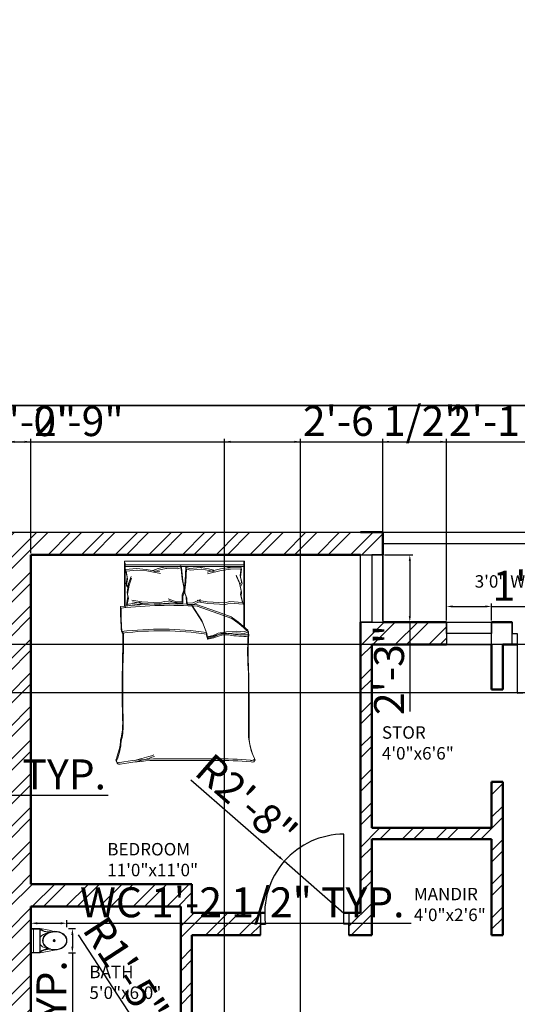
# Model space of a CAD drawing. Units: inches. Extents: x 1990 to 2869, y 1755 to 2533.
# Tile 5 of 6: x 2415 to 2615, y 2139 to 2533. Entities that reach past the tile are written whole.
import ezdxf

# ---------------------------------------------------------------- set-up
doc = ezdxf.new("R2010")
doc.units = ezdxf.units.IN
for name, color, linetype, lineweight in [('A-ANNO-DIMS', 171, 'Continuous', 18), ('A-ANNO-TTLB', 7, 'Continuous', 35), ('A-AREA-IDEN', 7, 'Continuous', 18), ('A-DOOR', 11, 'Continuous', 25), ('A-FLOR-FIXT', 9, 'Continuous', 20), ('A-FURN', 8, 'Continuous', 18), ('A-GLAZ', 121, 'Continuous', 25), ('A-WALL', 7, 'Continuous', 50), ('A-WALL-SITE', 7, 'Continuous', 30)]:
    doc.layers.add(name, color=color, linetype=linetype, lineweight=lineweight)
doc.layers.add('A-WALL-PATT', color=215, linetype='Continuous', lineweight=13, true_color=0xa953a0)
doc.styles.get("Standard").update_dxf_attribs({"font": 'arial.ttf'})
doc.dimstyles.new('ISO-25', dxfattribs={"dimtxt": 12, "dimasz": 2.5, "dimexe": 1.25, "dimexo": 0.625, "dimtad": 1, "dimdec": 0, "dimlunit": 3, "dimtxsty": 'Standard', "dimcen": 2.5, "dimadec": 0, "dimazin": 0, "dimtfac": 1, "dimtdec": 0, "dimtmove": 0, "dimatfit": 3, "dimfxl": 1, "dimarcsym": 0})

# ---------------------------------------------------------------- blocks, each defined once
blk = doc.blocks.new('A$C31115884')
for p, q in [((283, 498), (223, 498)), ((258, 466), (258, 523)), ((0, 200), (0, 0)), ((520, 200), (0, 200)), ((510, 54), (0, 54)), ((10, 190), (10, 10)), ((510, 190), (10, 190)), ((10, 10), (510, 10)), ((510, 10), (510, 190)), ((520, 0), (520, 200)), ((0, 0), (520, 0))]:
    blk.add_line(p, q)
blk.add_circle((256, 496), 23.6)
for centre, radius, start, end in [((2778, -205), 2807, 165.4549, 171.7133), ((-295, 403), 365, 324.2091, 9.3499), ((-295, 403), 375, 324.2091, 9.3499), ((806, 403), 365, 170.6501, 215.7909), ((3237, 905), 2807, 188.2867, 194.5451), ((384, 406), 293, 190.2774, 224.1564), ((139, 406), 293, 315.8436, 2.6563), ((806, 403), 375, 179.2036, 215.7909)]:
    blk.add_arc(centre, radius, start, end)
blk.add_ellipse((256, 510), major_axis=(0, -261), ratio=0.772727)
blk.add_open_spline([(256, 259), (263, 259), (270, 260), (288, 262), (299, 265), (320, 273), (330, 278), (350, 291), (360, 299), (378, 316), (386, 326), (402, 347), (409, 358), (421, 383), (427, 395), (436, 422), (440, 436), (445, 465), (447, 480), (448, 509), (448, 524), (445, 553), (443, 568), (436, 596), (432, 610), (422, 636), (416, 649), (402, 672), (395, 683), (379, 703), (370, 712), (351, 728), (341, 735), (321, 746), (310, 751), (289, 757), (278, 759), (256, 761), (245, 761), (223, 757), (212, 754), (191, 746), (181, 741), (161, 728), (151, 720), (133, 703), (125, 693), (110, 672), (103, 660), (90, 636), (85, 623), (76, 596), (72, 582), (67, 553), (66, 538), (64, 509), (65, 494), (68, 465), (70, 450), (77, 422), (81, 408), (91, 382), (97, 370), (111, 346), (118, 335), (135, 316), (144, 307), (162, 291), (172, 284), (193, 273), (203, 269), (225, 262), (236, 260), (250, 259), (253, 259), (256, 259)], degree=3, knots=[0, 0, 0, 0, 0.110105, 0.110105, 0.285049, 0.285049, 0.459994, 0.459994, 0.634938, 0.634938, 0.809882, 0.809882, 0.984827, 0.984827, 1.159771, 1.159771, 1.334715, 1.334715, 1.50966, 1.50966, 1.684604, 1.684604, 1.859549, 1.859549, 2.034493, 2.034493, 2.209437, 2.209437, 2.384382, 2.384382, 2.559326, 2.559326, 2.73427, 2.73427, 2.909215, 2.909215, 3.084159, 3.084159, 3.259103, 3.259103, 3.434048, 3.434048, 3.608992, 3.608992, 3.783936, 3.783936, 3.958881, 3.958881, 4.133825, 4.133825, 4.30877, 4.30877, 4.483714, 4.483714, 4.658658, 4.658658, 4.833603, 4.833603, 5.008547, 5.008547, 5.183491, 5.183491, 5.358436, 5.358436, 5.53338, 5.53338, 5.708324, 5.708324, 5.883269, 5.883269, 6.058213, 6.058213, 6.233158, 6.233158, 6.283185, 6.283185, 6.283185, 6.283185])
blk = doc.blocks.new('*D13')
at = {"layer": 'A-ANNO-DIMS', "color": 0, "lineweight": -2, "transparency": 16777216}
for p, q in [((2586.47, 2292.68), (2586.47, 2299.57)), ((2588.97, 2298.32), (2601.97, 2298.32)), ((2604.47, 2292.68), (2604.47, 2299.57)), ((2604.47, 2298.32), (2638.99, 2298.32))]:
    blk.add_line(p, q, dxfattribs=at)
at = {"layer": 'A-ANNO-DIMS', "color": 0, "transparency": 16777216}
for points in [[(2588.97, 2298.74), (2588.97, 2297.9), (2586.47, 2298.32)], [(2601.97, 2298.74), (2601.97, 2297.9), (2604.47, 2298.32)]]:
    blk.add_solid(points, dxfattribs=at)
at = {"layer": 'Defpoints', "color": 0, "transparency": 16777216}
for p in [(2604.47, 2298.32), (2586.47, 2292.05), (2604.47, 2292.05)]:
    blk.add_point(p, dxfattribs=at)
at = {"layer": 'A-ANNO-DIMS', "color": 0, "transparency": 16777216, "insert": (2622.98, 2305.07), "char_height": 12, "attachment_point": 5}
blk.add_mtext('1\'-6"', dxfattribs=at)
blk = doc.blocks.new('*D14')
at = {"layer": 'A-ANNO-DIMS', "color": 0, "lineweight": -2, "transparency": 16777216}
for p, q in [((2561.6, 2319.05), (2573, 2319.05)), ((2571.75, 2316.55), (2571.75, 2294.55)), ((2561.6, 2292.05), (2573, 2292.05)), ((2571.75, 2292.05), (2571.75, 2256.2))]:
    blk.add_line(p, q, dxfattribs=at)
at = {"layer": 'A-ANNO-DIMS', "color": 0, "transparency": 16777216}
for points in [[(2571.33, 2316.55), (2572.17, 2316.55), (2571.75, 2319.05)], [(2571.33, 2294.55), (2572.17, 2294.55), (2571.75, 2292.05)]]:
    blk.add_solid(points, dxfattribs=at)
at = {"layer": 'Defpoints', "color": 0, "transparency": 16777216}
for p in [(2560.97, 2319.05), (2560.97, 2292.05), (2571.75, 2292.05)]:
    blk.add_point(p, dxfattribs=at)
at = {"layer": 'A-ANNO-DIMS', "color": 0, "transparency": 16777216, "insert": (2564.99, 2272.87), "char_height": 12, "attachment_point": 5, "rotation": 90}
blk.add_mtext('2\'-3"', dxfattribs=at)
blk = doc.blocks.new('BED-DOUBLE')
for p, q in [((3.47, 63.33), (3.47, 81.44)), ((3.47, 81.44), (51.49, 81.44)), ((3.47, 79.91), (51.27, 79.91)), ((3.48, 63.33), (3.48, 81.44)), ((3.48, 79.91), (51.27, 79.91)), ((3.7, 62.69), (3.7, 80.8)), ((3.7, 62.69), (3.7, 80.8)), ((3.7, 79.27), (51.49, 79.27)), ((3.7, 79.27), (51.49, 79.27)), ((16.88, 78.42), (19.77, 79.14)), ((16.88, 78.42), (19.77, 79.14)), ((19.77, 79.14), (20.09, 79.14)), ((19.77, 79.14), (20.09, 79.14)), ((20.09, 79.14), (24.54, 78.99)), ((20.09, 79.14), (24.54, 78.99)), ((24.54, 78.99), (25.98, 79.57)), ((24.54, 78.99), (25.98, 79.57)), ((24.77, 78.36), (26.21, 78.93)), ((24.77, 78.36), (26.21, 78.93)), ((25.98, 79.57), (26.56, 74.22)), ((25.98, 79.57), (26.56, 74.22)), ((26.21, 78.93), (26.79, 73.58)), ((26.21, 78.93), (26.79, 73.58)), ((27.98, 78.95), (27.73, 73.58)), ((27.98, 78.95), (27.73, 73.58)), ((29.46, 78.46), (27.98, 78.95)), ((29.46, 78.46), (27.98, 78.95)), ((50.11, 78.89), (44.71, 78.98)), ((44.71, 78.98), (45.71, 78.9)), ((50.11, 78.89), (44.71, 78.98)), ((44.71, 78.98), (45.71, 78.9)), ((51.27, 81.44), (51.27, 54.83)), ((51.27, 81.44), (51.27, 54.83)), ((51.49, 81.44), (51.49, 80.8)), ((51.49, 80.8), (51.49, 54.19)), ((51.49, 80.8), (51.49, 54.19)), ((3.89, 78.13), (4.47, 74.95)), ((3.89, 78.13), (4.47, 74.95)), ((3.9, 78.11), (8.18, 78.43)), ((3.9, 78.11), (8.18, 78.43)), ((4.12, 77.49), (4.7, 74.31)), ((4.12, 77.49), (4.7, 74.31)), ((4.13, 77.47), (8.41, 77.8)), ((4.13, 77.47), (8.41, 77.8)), ((5.05, 72.49), (6.06, 75.24)), ((5.05, 72.49), (6.06, 75.24)), ((8.18, 78.43), (8.28, 78.42)), ((8.18, 78.43), (8.28, 78.42)), ((8.28, 78.42), (12.11, 78.13)), ((8.28, 78.42), (12.11, 78.13)), ((8.41, 77.8), (8.51, 77.78)), ((8.41, 77.8), (8.51, 77.78)), ((8.51, 77.78), (12.34, 77.49)), ((8.51, 77.78), (12.34, 77.49)), ((12.11, 78.13), (17.6, 77.11)), ((12.11, 78.13), (17.6, 77.11)), ((12.34, 77.49), (17.83, 76.48)), ((12.34, 77.49), (17.83, 76.48)), ((14.85, 77.69), (16.88, 78.42)), ((14.85, 77.69), (16.88, 78.42)), ((15.08, 77.05), (17.11, 77.78)), ((15.08, 77.05), (17.11, 77.78)), ((17.11, 77.78), (20, 78.5)), ((17.11, 77.78), (20, 78.5)), ((20, 78.5), (20.32, 78.5)), ((20, 78.5), (20.32, 78.5)), ((20.32, 78.5), (24.77, 78.36)), ((20.32, 78.5), (24.77, 78.36)), ((28.21, 78.31), (27.96, 72.94)), ((28.2, 78.31), (27.96, 72.94)), ((29.68, 77.82), (28.2, 78.31)), ((29.68, 77.82), (28.21, 78.31)), ((33.88, 78.89), (29.46, 78.46)), ((33.88, 78.89), (29.46, 78.46)), ((34.11, 78.25), (29.68, 77.82)), ((34.11, 78.25), (29.68, 77.82)), ((34.2, 78.91), (33.88, 78.89)), ((34.2, 78.91), (33.88, 78.89)), ((34.43, 78.27), (34.11, 78.25)), ((34.43, 78.27), (34.11, 78.25)), ((37.14, 78.36), (34.2, 78.91)), ((37.13, 78.36), (34.2, 78.91)), ((37.36, 77.73), (34.43, 78.27)), ((37.36, 77.73), (34.43, 78.27)), ((41.91, 78.37), (36.49, 77.02)), ((41.91, 78.37), (36.49, 77.02)), ((42.14, 77.73), (36.72, 76.38)), ((42.14, 77.73), (36.72, 76.38)), ((39.2, 77.77), (37.13, 78.36)), ((39.2, 77.77), (37.14, 78.36)), ((39.43, 77.13), (37.36, 77.73)), ((39.43, 77.13), (37.36, 77.73)), ((45.71, 78.9), (41.91, 78.37)), ((45.71, 78.9), (41.91, 78.37)), ((45.94, 78.26), (42.14, 77.73)), ((45.94, 78.26), (42.14, 77.73)), ((50.34, 78.25), (44.94, 78.34)), ((44.94, 78.34), (45.94, 78.26)), ((50.34, 78.25), (44.94, 78.34)), ((44.94, 78.34), (45.94, 78.26)), ((49.31, 73.19), (48.13, 75.86)), ((49.31, 73.19), (48.13, 75.86)), ((49.54, 72.55), (48.36, 75.23)), ((49.54, 72.55), (48.36, 75.23)), ((50.11, 78.89), (49.73, 75.68)), ((50.11, 78.89), (49.73, 75.68)), ((49.73, 75.68), (50.33, 73.1)), ((49.73, 75.68), (50.33, 73.1)), ((50.34, 78.25), (49.96, 75.04)), ((50.34, 78.25), (49.96, 75.04)), ((49.96, 75.04), (50.56, 72.47)), ((49.96, 75.04), (50.56, 72.47)), ((4.47, 74.95), (4.04, 72.34)), ((4.47, 74.95), (4.04, 72.34)), ((4.04, 72.34), (4.62, 71.33)), ((4.04, 72.34), (4.62, 71.33)), ((4.7, 74.31), (4.27, 71.7)), ((4.7, 74.31), (4.27, 71.7)), ((4.27, 71.7), (4.85, 70.69)), ((4.27, 71.7), (4.85, 70.69)), ((4.47, 68.87), (5.05, 72.49)), ((4.47, 68.87), (5.05, 72.49)), ((4.7, 68.23), (5.28, 71.85)), ((4.7, 68.23), (5.28, 71.85)), ((5.28, 71.85), (6.29, 74.6)), ((5.28, 71.85), (6.29, 74.6)), ((26.56, 74.22), (27.14, 71.04)), ((26.56, 74.22), (27.14, 71.04)), ((26.79, 73.58), (27.37, 70.4)), ((26.79, 73.58), (27.37, 70.4)), ((27.14, 71.04), (27.14, 69.74)), ((27.14, 71.04), (27.14, 69.74)), ((27.73, 73.58), (27.35, 70.37)), ((27.73, 73.58), (27.35, 70.37)), ((27.96, 72.94), (27.58, 69.73)), ((27.96, 72.94), (27.58, 69.73)), ((50.11, 69.61), (49.31, 73.19)), ((50.11, 69.61), (49.31, 73.19)), ((50.34, 68.98), (49.54, 72.55)), ((50.34, 68.98), (49.54, 72.55)), ((50.33, 73.1), (49.81, 72.06)), ((50.33, 73.1), (49.81, 72.06)), ((50.56, 72.47), (50.04, 71.42)), ((50.56, 72.47), (50.04, 71.42)), ((4.18, 64.1), (4.76, 67.28)), ((4.18, 64.1), (4.76, 67.28)), ((4.76, 67.28), (4.47, 68.87)), ((4.76, 67.28), (4.47, 68.87)), ((4.99, 66.64), (4.7, 68.23)), ((4.99, 66.64), (4.7, 68.23)), ((27.14, 69.74), (26.56, 67.86)), ((27.14, 69.74), (26.56, 67.86)), ((26.56, 67.86), (26.56, 65.18)), ((26.56, 67.86), (26.56, 65.18)), ((27.37, 69.1), (26.79, 67.22)), ((27.37, 69.1), (26.79, 67.22)), ((26.79, 67.22), (26.79, 64.54)), ((26.79, 67.22), (26.79, 64.54)), ((27.35, 70.37), (27.44, 69.07)), ((27.35, 70.37), (27.44, 69.07)), ((27.37, 70.4), (27.37, 69.1)), ((27.37, 70.4), (27.37, 69.1)), ((27.44, 69.07), (28.13, 67.23)), ((27.44, 69.07), (28.13, 67.23)), ((27.58, 69.73), (27.66, 68.43)), ((27.58, 69.73), (27.66, 68.43)), ((27.66, 68.43), (28.36, 66.59)), ((27.66, 68.43), (28.36, 66.59)), ((28.13, 67.23), (28.3, 64.55)), ((28.13, 67.23), (28.3, 64.55)), ((49.92, 68.01), (50.11, 69.61)), ((49.92, 68.01), (50.11, 69.61)), ((50.7, 64.87), (49.92, 68.01)), ((50.7, 64.87), (49.92, 68.01)), ((50.15, 67.37), (50.34, 68.98)), ((50.15, 67.37), (50.34, 68.98)), ((50.93, 64.23), (50.15, 67.37)), ((50.93, 64.23), (50.15, 67.37)), ((9.28, 64.82), (4.18, 64.1)), ((9.28, 64.82), (4.18, 64.1)), ((4.41, 63.46), (4.99, 66.64)), ((4.41, 63.46), (4.99, 66.64)), ((9.51, 64.19), (4.41, 63.46)), ((9.51, 64.19), (4.41, 63.46)), ((6.38, 65.81), (10.41, 65.15)), ((6.38, 65.81), (10.41, 65.15)), ((6.61, 65.18), (10.64, 64.51)), ((6.61, 65.18), (10.64, 64.51)), ((10.41, 65.15), (9.28, 64.82)), ((10.41, 65.15), (9.28, 64.82)), ((10.64, 64.51), (9.51, 64.19)), ((10.64, 64.51), (9.51, 64.19)), ((10.41, 65.15), (17.42, 64.72)), ((10.41, 65.15), (17.42, 64.72)), ((10.64, 64.51), (17.65, 64.08)), ((10.64, 64.51), (17.65, 64.08)), ((17.42, 64.72), (19.38, 65.27)), ((17.42, 64.72), (19.38, 65.27)), ((17.65, 64.08), (19.61, 64.63)), ((17.65, 64.08), (19.61, 64.63)), ((19.38, 65.27), (24.52, 64.87)), ((19.38, 65.27), (24.52, 64.87)), ((19.61, 64.63), (24.74, 64.23)), ((19.61, 64.63), (24.74, 64.23)), ((24.1, 65.18), (20.96, 66.27)), ((24.1, 65.18), (20.96, 66.27)), ((24.33, 64.54), (21.19, 65.63)), ((24.33, 64.54), (21.19, 65.63)), ((26.56, 65.18), (24.1, 65.18)), ((26.56, 65.18), (24.1, 65.18)), ((26.79, 64.54), (24.33, 64.54)), ((26.79, 64.54), (24.33, 64.54)), ((28.3, 64.55), (30.75, 64.7)), ((28.3, 64.55), (30.75, 64.7)), ((28.36, 66.59), (28.53, 63.91)), ((28.36, 66.59), (28.53, 63.91)), ((28.53, 63.91), (30.98, 64.06)), ((28.53, 63.91), (30.98, 64.06)), ((30.26, 64.06), (34.45, 57.57)), ((30.26, 64.06), (34.45, 57.57)), ((30.49, 63.42), (34.68, 56.93)), ((30.49, 63.42), (34.68, 56.93)), ((30.75, 64.7), (33.82, 65.99)), ((30.75, 64.7), (33.82, 65.99)), ((30.98, 64.06), (34.05, 65.35)), ((30.98, 64.06), (34.05, 65.35)), ((40.64, 61.13), (32.31, 64.06)), ((40.64, 61.13), (32.31, 64.06)), ((40.87, 60.49), (32.53, 63.42)), ((40.87, 60.49), (32.53, 63.42)), ((32.56, 65.81), (36.6, 65.15)), ((32.56, 65.81), (36.6, 65.15)), ((32.79, 65.18), (36.82, 64.51)), ((32.79, 65.18), (36.82, 64.51)), ((36.6, 65.15), (43.61, 64.72)), ((36.6, 65.15), (43.61, 64.72)), ((36.82, 64.51), (43.83, 64.08)), ((36.82, 64.51), (43.83, 64.08)), ((43.61, 64.72), (45.57, 65.27)), ((43.61, 64.72), (45.57, 65.27)), ((43.83, 64.08), (45.79, 64.63)), ((43.83, 64.08), (45.79, 64.63)), ((45.57, 65.27), (50.7, 64.87)), ((45.57, 65.27), (50.7, 64.87)), ((45.79, 64.63), (50.93, 64.23)), ((45.79, 64.63), (50.93, 64.23)), ((46.22, 59.11), (40.64, 61.13)), ((46.22, 59.11), (40.64, 61.13)), ((46.45, 58.48), (40.87, 60.49)), ((46.45, 58.48), (40.87, 60.49)), ((34.45, 57.57), (36.15, 53.08)), ((34.45, 57.57), (36.15, 53.08)), ((34.68, 56.93), (36.38, 52.44)), ((34.68, 56.93), (36.38, 52.44)), ((49.16, 56.95), (46.22, 59.11)), ((49.16, 56.95), (46.22, 59.11)), ((49.39, 56.31), (46.45, 58.48)), ((49.39, 56.31), (46.45, 58.48)), ((52.87, 53.7), (49.16, 56.95)), ((52.87, 53.7), (49.16, 56.95)), ((53.1, 53.06), (49.39, 56.31)), ((53.1, 53.06), (49.39, 56.31)), ((36.15, 53.08), (36.46, 51.07)), ((36.15, 53.08), (36.46, 51.07)), ((36.38, 52.44), (36.69, 50.43)), ((36.38, 52.44), (36.69, 50.43)), ((36.46, 51.07), (38.94, 51.69)), ((36.46, 51.07), (38.94, 51.69)), ((38.94, 51.69), (40.95, 52.61)), ((38.94, 51.69), (40.95, 52.61)), ((39.17, 51.05), (41.18, 51.97)), ((39.17, 51.05), (41.18, 51.97)), ((40.95, 52.61), (44.36, 53.08)), ((40.95, 52.61), (44.36, 53.08)), ((41.18, 51.97), (44.59, 52.44)), ((41.18, 51.97), (44.59, 52.44)), ((44.36, 53.08), (48.23, 53.39)), ((44.36, 53.08), (48.23, 53.39)), ((44.59, 52.44), (48.46, 52.75)), ((44.59, 52.44), (48.46, 52.75)), ((48.23, 53.39), (51.33, 53.08)), ((48.23, 53.39), (51.33, 53.08)), ((48.46, 52.75), (51.56, 52.44)), ((48.46, 52.75), (51.56, 52.44)), ((51.33, 53.08), (52.87, 53.7)), ((51.33, 53.08), (52.87, 53.7)), ((51.56, 52.44), (53.1, 53.06)), ((51.56, 52.44), (53.1, 53.06)), ((52.95, 51.95), (52.87, 53.7, 3.87)), ((52.95, 51.95), (52.87, 53.7, 3.87)), ((53.18, 51.31), (53.1, 53.06, 3.87)), ((53.18, 51.31), (53.1, 53.06, 3.87)), ((36.69, 50.43), (39.17, 51.05)), ((36.69, 50.43), (39.17, 51.05)), ((15.06, 2.2), (39.68, 2.2)), ((15.06, 2.2), (39.68, 2.2)), ((15.29, 1.56), (39.91, 1.56)), ((15.29, 1.56), (39.91, 1.56))]:
    blk.add_line(p, q)
for centre, radius, start, end in [((85.16, 61.35), 83.31, 178.7218, 185.604), ((85.16, 61.35), 83.31, 178.7218, 185.604), ((21.36, -100.61), 164.97, 86.0865, 96.7821), ((21.36, -100.61), 164.97, 86.0865, 96.7821), ((21.59, -101.25), 164.97, 86.0865, 96.7821), ((21.59, -101.25), 164.97, 86.0865, 96.7821), ((85.39, 60.71), 83.31, 178.7218, 185.604), ((85.39, 60.71), 83.31, 178.7218, 185.604), ((17.76, -74.87), 129.02, 81.7845, 96.9006), ((17.76, -74.87), 129.02, 81.7845, 96.9006), ((17.98, -75.51), 129.02, 81.7845, 96.9006), ((17.98, -75.51), 129.02, 81.7845, 96.9006), ((-167.31, 50.27), 170.11, 358.4762, 1.0082), ((-167.31, 50.27), 170.11, 358.4762, 1.0082), ((-167.08, 49.63), 170.11, 358.4762, 1.0082), ((-167.08, 49.63), 170.11, 358.4762, 1.0082), ((31.15, 79.96), 29.65, 280.6617, 289.8806), ((31.15, 79.96), 29.65, 280.6617, 289.8806), ((31.38, 79.32), 29.65, 280.6617, 289.8806), ((31.38, 79.32), 29.65, 280.6617, 289.8806), ((43.74, 46.38), 6.22, 78.6608, 113.7384), ((43.74, 46.38), 6.22, 78.6608, 113.7384), ((43.97, 45.74), 6.22, 78.6608, 113.7384), ((43.97, 45.74), 6.22, 78.6608, 113.7384), ((51.33, 88.1), 36.18, 259.8763, 272.5657), ((51.33, 88.1), 36.18, 259.8763, 272.5657), ((51.56, 87.46), 36.18, 259.8763, 272.5657), ((51.56, 87.46), 36.18, 259.8763, 272.5657), ((182.27, 45.13), 129.5, 176.9791, 183.8365), ((182.27, 45.13), 129.5, 176.9791, 183.8365), ((182.49, 44.49), 129.5, 176.9791, 183.8365), ((182.49, 44.49), 129.5, 176.9791, 183.8365), ((36.64, 51), 0.185, 160.2464, 271.1377), ((36.64, 51), 0.185, 160.2464, 271.1377), ((36.86, 50.36), 0.185, 160.2464, 271.1377), ((36.86, 50.36), 0.185, 160.2464, 271.1377), ((484.82, 30.83), 482.31, 178.2277, 181.7185), ((484.82, 30.83), 482.31, 178.2277, 181.7185), ((485.05, 30.19), 482.31, 178.2277, 181.7185), ((485.05, 30.19), 482.31, 178.2277, 181.7185), ((-4508.74, 13.62), 4561.86, 0.00217, 0.28689), ((-4508.74, 13.62), 4561.86, 0.00217, 0.28689), ((-4508.52, 12.98), 4561.86, 0.00217, 0.28689), ((-4508.52, 12.98), 4561.86, 0.00217, 0.28689), ((-26.9, 16.93), 29.63, 346.0648, 358.9113), ((-26.9, 16.93), 29.63, 346.0648, 358.9113), ((-26.67, 16.29), 29.63, 346.0648, 358.9113), ((-26.67, 16.29), 29.63, 346.0648, 358.9113), ((76.16, 12.78), 23.07, 177.4714, 206.4681), ((76.16, 12.78), 23.07, 177.4714, 206.4681), ((76.39, 12.14), 23.07, 177.4714, 206.4681), ((76.39, 12.14), 23.07, 177.4714, 206.4681), ((-21.66, 11.17), 23.56, 337.9751, 356.652), ((-21.66, 11.17), 23.56, 337.9751, 356.652), ((-21.43, 10.53), 23.56, 337.9751, 356.652), ((-21.43, 10.53), 23.56, 337.9751, 356.652), ((1.09, 1.73), 1.09, 146.1736, 293.4781), ((1.09, 1.73), 1.09, 146.1736, 293.4781), ((1.32, 1.09), 1.09, 146.1736, 293.4781), ((1.32, 1.09), 1.09, 146.1736, 293.4781), ((21.43, -119.39), 121.76, 92.9958, 99.4091), ((21.43, -119.39), 121.76, 92.9958, 99.4091), ((21.66, -120.03), 121.76, 92.9958, 99.4091), ((21.65, -120.03), 121.76, 92.9958, 99.4091), ((-17.22, 105.15), 106.46, 283.3832, 287.7053), ((-17.22, 105.15), 106.46, 283.3832, 287.7053), ((-16.99, 104.52), 106.46, 283.3832, 287.7053), ((-16.99, 104.52), 106.46, 283.3832, 287.7053), ((41.15, -130.83), 133.04, 84.4998, 90.6351), ((41.15, -130.83), 133.04, 84.4998, 90.6351), ((41.38, -131.47), 133.04, 84.4998, 90.6351), ((41.38, -131.47), 133.04, 84.4998, 90.6351), ((54.41, 2.57), 1.1, 242.6588, 356.02), ((54.41, 2.57), 1.1, 242.6588, 356.02), ((54.64, 1.93), 1.1, 242.6588, 356.02), ((54.64, 1.93), 1.1, 242.6588, 356.02)]:
    blk.add_arc(centre, radius, start, end)
blk = doc.blocks.new('WIN-18IN')
for p, q in [((0, 4.5), (0, 9)), ((0, 9), (0, 0)), ((0, 9), (18, 9)), ((18, 0), (18, 9)), ((18, 9), (18, 4.5)), ((18, 4.5), (0, 4.5)), ((0, 0), (18, 0))]:
    blk.add_line(p, q)
blk = doc.blocks.new('*D20')
at = {"layer": 'A-ANNO-DIMS', "color": 0, "lineweight": -2, "transparency": 16777216}
for p, q in [((2385.7, 2316.5), (2385.7, 2533.49)), ((2374.09, 2316.5), (2386.95, 2316.5)), ((2385.7, 2237.45), (2385.7, 2314)), ((2374.09, 2234.95), (2386.95, 2234.95))]:
    blk.add_line(p, q, dxfattribs=at)
at = {"layer": 'A-ANNO-DIMS', "color": 0, "transparency": 16777216}
for points in [[(2385.29, 2314), (2386.12, 2314), (2385.7, 2316.5)], [(2385.29, 2237.45), (2386.12, 2237.45), (2385.7, 2234.95)]]:
    blk.add_solid(points, dxfattribs=at)
at = {"layer": 'Defpoints', "color": 0, "transparency": 16777216}
for p in [(2373.47, 2316.5), (2385.7, 2316.5), (2373.47, 2234.95)]:
    blk.add_point(p, dxfattribs=at)
at = {"layer": 'A-ANNO-DIMS', "color": 0, "transparency": 16777216, "insert": (2378.87, 2426.24), "char_height": 12, "attachment_point": 5, "rotation": 90}
blk.add_mtext('DOUBLE BED 6\'-9 1/2" TYP.', dxfattribs=at)
blk = doc.blocks.new('*D21')
at = {"layer": 'A-ANNO-DIMS', "color": 0, "lineweight": -2, "transparency": 16777216}
for p, q in [((2317.65, 2234.33), (2317.65, 2221.47)), ((2373.47, 2234.33), (2373.47, 2221.47)), ((2320.15, 2222.72), (2370.97, 2222.72)), ((2373.47, 2222.72), (2450.85, 2222.72))]:
    blk.add_line(p, q, dxfattribs=at)
at = {"layer": 'A-ANNO-DIMS', "color": 0, "transparency": 16777216}
for points in [[(2320.15, 2223.14), (2320.15, 2222.31), (2317.65, 2222.72)], [(2370.97, 2223.14), (2370.97, 2222.31), (2373.47, 2222.72)]]:
    blk.add_solid(points, dxfattribs=at)
at = {"layer": 'Defpoints', "color": 0, "transparency": 16777216}
for p in [(2317.65, 2234.95), (2373.47, 2234.95), (2373.47, 2222.72)]:
    blk.add_point(p, dxfattribs=at)
at = {"layer": 'A-ANNO-DIMS', "color": 0, "transparency": 16777216, "insert": (2413.41, 2229.47), "char_height": 12, "attachment_point": 5}
blk.add_mtext('4\'-8" TYP.', dxfattribs=at)
blk = doc.blocks.new('*D22')
at = {"layer": 'A-ANNO-DIMS', "color": 0, "lineweight": -2, "transparency": 16777216}
for p, q in [((2419.97, 2169.82), (2419.97, 2172.61)), ((2422.47, 2171.36), (2431.91, 2171.36)), ((2434.41, 2169.82), (2434.41, 2172.61)), ((2434.41, 2171.36), (2572.34, 2171.36))]:
    blk.add_line(p, q, dxfattribs=at)
at = {"layer": 'A-ANNO-DIMS', "color": 0, "transparency": 16777216}
for points in [[(2422.47, 2171.77), (2422.47, 2170.94), (2419.97, 2171.36)], [(2431.91, 2171.77), (2431.91, 2170.94), (2434.41, 2171.36)]]:
    blk.add_solid(points, dxfattribs=at)
at = {"layer": 'Defpoints', "color": 0, "transparency": 16777216}
for p in [(2434.41, 2171.36), (2419.97, 2169.19), (2434.41, 2169.19)]:
    blk.add_point(p, dxfattribs=at)
at = {"layer": 'A-ANNO-DIMS', "color": 0, "transparency": 16777216, "insert": (2504.62, 2178.19), "char_height": 12, "attachment_point": 5}
blk.add_mtext('WC 1\'-2 1/2" TYP.', dxfattribs=at)
blk = doc.blocks.new('*D23')
at = {"layer": 'A-ANNO-DIMS', "color": 0, "lineweight": -2, "transparency": 16777216}
for p, q in [((2435.03, 2169.19), (2437.82, 2169.19)), ((2436.57, 2166.69), (2436.57, 2161.95)), ((2435.03, 2159.45), (2437.82, 2159.45)), ((2436.57, 2159.45), (2436.57, 2054.59))]:
    blk.add_line(p, q, dxfattribs=at)
at = {"layer": 'A-ANNO-DIMS', "color": 0, "transparency": 16777216}
for points in [[(2436.15, 2166.69), (2436.99, 2166.69), (2436.57, 2169.19)], [(2436.15, 2161.95), (2436.99, 2161.95), (2436.57, 2159.45)]]:
    blk.add_solid(points, dxfattribs=at)
at = {"layer": 'Defpoints', "color": 0, "transparency": 16777216}
for p in [(2434.41, 2169.19), (2434.41, 2159.45), (2436.57, 2159.45)]:
    blk.add_point(p, dxfattribs=at)
at = {"layer": 'A-ANNO-DIMS', "color": 0, "transparency": 16777216, "insert": (2429.74, 2105.77), "char_height": 12, "attachment_point": 5, "rotation": 90}
blk.add_mtext('0\'-9 1/2" TYP.', dxfattribs=at)
blk = doc.blocks.new('*D32')
at = {"layer": 'A-ANNO-DIMS', "color": 0, "lineweight": -2, "transparency": 16777216}
for p, q in [((2497.49, 1974.68), (2497.49, 2365.55)), ((2499.99, 2364.3), (2525.47, 2364.3)), ((2527.97, 1974.68), (2527.97, 2365.55)), ((2527.97, 2364.3), (2591.79, 2364.3))]:
    blk.add_line(p, q, dxfattribs=at)
at = {"layer": 'A-ANNO-DIMS', "color": 0, "transparency": 16777216}
for points in [[(2499.99, 2364.72), (2499.99, 2363.88), (2497.49, 2364.3)], [(2525.47, 2364.72), (2525.47, 2363.88), (2527.97, 2364.3)]]:
    blk.add_solid(points, dxfattribs=at)
at = {"layer": 'Defpoints', "color": 0, "transparency": 16777216}
for p in [(2527.97, 2364.3), (2497.49, 1974.05), (2527.97, 1974.05)]:
    blk.add_point(p, dxfattribs=at)
at = {"layer": 'A-ANNO-DIMS', "color": 0, "transparency": 16777216, "insert": (2561.13, 2371.13), "char_height": 12, "attachment_point": 5}
blk.add_mtext('2\'-6 1/2"', dxfattribs=at)
blk = doc.blocks.new('*D36')
at = {"layer": 'A-ANNO-DIMS', "color": 0, "lineweight": -2, "transparency": 16777216}
for p, q in [((2716.35, 2283.05), (2016.97, 2283.05)), ((2018.22, 2280.55), (2018.22, 2266.18)), ((2716.35, 2263.68), (2016.97, 2263.68)), ((2018.22, 2263.68), (2018.22, 2201.19))]:
    blk.add_line(p, q, dxfattribs=at)
at = {"layer": 'A-ANNO-DIMS', "color": 0, "transparency": 16777216}
for points in [[(2017.8, 2280.55), (2018.64, 2280.55), (2018.22, 2283.05)], [(2017.8, 2266.18), (2018.64, 2266.18), (2018.22, 2263.68)]]:
    blk.add_solid(points, dxfattribs=at)
at = {"layer": 'Defpoints', "color": 0, "transparency": 16777216}
for p in [(2716.97, 2283.05), (2018.22, 2263.68), (2716.97, 2263.68)]:
    blk.add_point(p, dxfattribs=at)
at = {"layer": 'A-ANNO-DIMS', "color": 0, "transparency": 16777216, "insert": (2011.39, 2231.19), "char_height": 12, "attachment_point": 5, "rotation": 90}
blk.add_mtext('1\'-7 1/2"', dxfattribs=at)
blk = doc.blocks.new('*D38')
at = {"layer": 'A-ANNO-DIMS', "color": 0, "lineweight": -2, "transparency": 16777216}
for p, q in [((2560.97, 2292.68), (2560.97, 2365.55)), ((2563.47, 2364.3), (2583.97, 2364.3)), ((2586.47, 2292.68), (2586.47, 2365.55)), ((2586.47, 2364.3), (2650.29, 2364.3))]:
    blk.add_line(p, q, dxfattribs=at)
at = {"layer": 'A-ANNO-DIMS', "color": 0, "transparency": 16777216}
for points in [[(2563.47, 2364.72), (2563.47, 2363.88), (2560.97, 2364.3)], [(2583.97, 2364.72), (2583.97, 2363.88), (2586.47, 2364.3)]]:
    blk.add_solid(points, dxfattribs=at)
at = {"layer": 'Defpoints', "color": 0, "transparency": 16777216}
for p in [(2586.47, 2364.3), (2560.97, 2292.05), (2586.47, 2292.05)]:
    blk.add_point(p, dxfattribs=at)
at = {"layer": 'A-ANNO-DIMS', "color": 0, "transparency": 16777216, "insert": (2619.63, 2371.13), "char_height": 12, "attachment_point": 5}
blk.add_mtext('2\'-1 1/2"', dxfattribs=at)
blk = doc.blocks.new('*D40')
at = {"layer": 'A-ANNO-DIMS', "color": 0, "lineweight": -2, "transparency": 16777216}
for p, q in [((2410.97, 2319.68), (2410.97, 2365.55)), ((2413.47, 2364.3), (2417.47, 2364.3)), ((2419.97, 2319.68), (2419.97, 2365.55)), ((2419.97, 2364.3), (2455.62, 2364.3))]:
    blk.add_line(p, q, dxfattribs=at)
at = {"layer": 'A-ANNO-DIMS', "color": 0, "transparency": 16777216}
for points in [[(2413.47, 2364.72), (2413.47, 2363.88), (2410.97, 2364.3)], [(2417.47, 2364.72), (2417.47, 2363.88), (2419.97, 2364.3)]]:
    blk.add_solid(points, dxfattribs=at)
at = {"layer": 'Defpoints', "color": 0, "transparency": 16777216}
for p in [(2419.97, 2364.3), (2410.97, 2319.05), (2419.97, 2319.05)]:
    blk.add_point(p, dxfattribs=at)
at = {"layer": 'A-ANNO-DIMS', "color": 0, "transparency": 16777216, "insert": (2439.05, 2371.05), "char_height": 12, "attachment_point": 5}
blk.add_mtext('0\'-9"', dxfattribs=at)
blk = doc.blocks.new('*D48')
at = {"layer": 'A-ANNO-DIMS', "color": 0, "lineweight": -2, "transparency": 16777216}
for p, q in [((2054.47, 2328.68), (2054.47, 2365.55)), ((2056.97, 2364.3), (2773.97, 2364.3)), ((2776.47, 2328.68), (2776.47, 2365.55))]:
    blk.add_line(p, q, dxfattribs=at)
at = {"layer": 'A-ANNO-DIMS', "color": 0, "transparency": 16777216}
for points in [[(2056.97, 2364.72), (2056.97, 2363.88), (2054.47, 2364.3)], [(2773.97, 2364.72), (2773.97, 2363.88), (2776.47, 2364.3)]]:
    blk.add_solid(points, dxfattribs=at)
at = {"layer": 'Defpoints', "color": 0, "transparency": 16777216}
for p in [(2776.47, 2364.3), (2054.47, 2328.05), (2776.47, 2328.05)]:
    blk.add_point(p, dxfattribs=at)
at = {"layer": 'A-ANNO-DIMS', "color": 0, "transparency": 16777216, "insert": (2415.47, 2371.05), "char_height": 12, "attachment_point": 5}
blk.add_mtext('60\'-2"', dxfattribs=at)
blk = doc.blocks.new('*D55')
at = {"layer": 'A-ANNO-DIMS', "color": 0, "lineweight": -2, "transparency": 16777216}
for p, q in [((2484.09, 2228.87), (2519.57, 2197.84)), ((2545.37, 2175.28), (2521.45, 2196.2))]:
    blk.add_line(p, q, dxfattribs=at)
at = {"layer": 'A-ANNO-DIMS', "color": 0, "transparency": 16777216}
blk.add_solid([(2519.84, 2198.16), (2519.29, 2197.53), (2521.45, 2196.2)], dxfattribs=at)
at = {"layer": 'Defpoints', "color": 0, "transparency": 16777216}
for p in [(2521.45, 2196.2), (2545.37, 2175.28)]:
    blk.add_point(p, dxfattribs=at)
at = {"layer": 'A-ANNO-DIMS', "color": 0, "transparency": 16777216, "insert": (2505.34, 2219.26), "char_height": 12, "attachment_point": 5, "rotation": 318.824}
blk.add_mtext('R2\'-8"', dxfattribs=at)
blk = doc.blocks.new('*D60')
at = {"layer": 'A-ANNO-DIMS', "color": 0, "lineweight": -2, "transparency": 16777216}
for p, q in [((2438.87, 2166.74), (2464.62, 2127.26)), ((2475.32, 2110.84), (2465.98, 2125.16))]:
    blk.add_line(p, q, dxfattribs=at)
at = {"layer": 'A-ANNO-DIMS', "color": 0, "transparency": 16777216}
blk.add_solid([(2464.97, 2127.48), (2464.27, 2127.03), (2465.98, 2125.16)], dxfattribs=at)
at = {"layer": 'Defpoints', "color": 0, "transparency": 16777216}
for p in [(2465.98, 2125.16), (2475.32, 2110.84)]:
    blk.add_point(p, dxfattribs=at)
at = {"layer": 'A-ANNO-DIMS', "color": 0, "transparency": 16777216, "insert": (2456.72, 2151.73), "char_height": 12, "attachment_point": 5, "rotation": 303.1079}
blk.add_mtext('R1\'-5"', dxfattribs=at)

msp = doc.modelspace()

# ---------------------------------------------------------------- hatches: boundary and pattern name
at = {"layer": 'A-WALL-PATT'}
h = msp.add_hatch(dxfattribs=at)
h.set_pattern_fill('ANSI32', color=256)
h.paths.add_polyline_path([(2193.46, 2287.55), (2131.97, 2287.55), (2131.97, 2278.55), (2193.46, 2278.55)])
h.paths.add_polyline_path([(2113.97, 2278.55), (2113.97, 2287.55), (2104.97, 2287.55), (2104.97, 2257.5), (2113.97, 2257.5)])
h.paths.add_polyline_path([(2113.97, 2205), (2104.97, 2205), (2104.97, 2166.55), (2140.97, 2166.55), (2140.97, 2160.48), (2149.97, 2160.48), (2149.97, 2166.55), (2170.14, 2166.55), (2170.14, 2175.55), (2113.97, 2175.55)])
h.paths.add_polyline_path([(2278.97, 2287.55), (2244.47, 2287.55), (2244.47, 2278.55), (2274.47, 2278.55), (2274.47, 2200.55), (2226.47, 2200.55), (2226.47, 2219.37), (2221.97, 2219.37), (2221.97, 2175.55), (2221.97, 2166.55), (2226.47, 2166.55), (2226.47, 2196.05), (2274.47, 2196.05), (2274.47, 2166.55), (2284.01, 2166.55), (2284.01, 2171.05), (2284.01, 2175.55), (2278.97, 2175.55), (2278.97, 2278.55)])
h.paths.add_polyline_path([(2226.47, 2283.05), (2226.47, 2287.55), (2217.66, 2287.55), (2217.66, 2283.05), (2217.66, 2278.55), (2221.97, 2278.55), (2221.97, 2255.21), (2226.47, 2255.21), (2226.47, 2278.55)])
h.paths.add_polyline_path([(2560.97, 2328.05), (2551.97, 2328.05), (2269.97, 2328.05), (2269.97, 2319.05), (2278.97, 2319.05), (2410.97, 2319.05), (2410.97, 2187.05), (2346.47, 2187.05), (2346.47, 2175.55), (2319.77, 2175.55), (2319.77, 2166.55), (2346.47, 2166.55), (2346.47, 2128.22), (2350.97, 2128.22), (2350.97, 2178.05), (2410.97, 2178.05), (2410.97, 2175.55), (2410.97, 2106.05), (2350.97, 2106.05), (2350.97, 2108.72), (2348.72, 2108.72), (2346.47, 2108.72), (2346.47, 2106.05), (2342.3, 2106.05), (2342.3, 2097.05), (2346.47, 2097.05), (2350.97, 2097.05), (2410.97, 2097.05), (2410.97, 1974.05), (2373.73, 1974.05), (2373.73, 1965.05), (2419.97, 1965.05), (2447.99, 1965.05), (2447.99, 1969.55), (2447.99, 1974.05), (2419.97, 1974.05), (2419.97, 2097.05), (2484.47, 2097.05), (2489.55, 2097.05), (2489.55, 2106.05), (2484.47, 2106.05), (2484.47, 2108.84), (2482.22, 2108.84), (2479.97, 2108.84), (2479.97, 2106.05), (2419.97, 2106.05), (2419.97, 2175.55), (2419.97, 2178.05), (2479.97, 2178.05), (2479.97, 2128.49), (2484.47, 2128.49), (2484.47, 2166.55), (2511.88, 2166.55), (2511.88, 2171.05), (2511.88, 2175.55), (2484.47, 2175.55), (2484.47, 2187.05), (2479.97, 2187.05), (2419.97, 2187.05), (2419.97, 2319.05), (2551.97, 2319.05), (2560.97, 2319.05)])
h.paths.add_polyline_path([(2586.47, 2292.05), (2560.97, 2292.05), (2551.97, 2292.05), (2551.97, 2175.55), (2547.37, 2175.55), (2547.37, 2166.55), (2556.47, 2166.55), (2556.47, 2175.55), (2556.47, 2205.05), (2604.47, 2205.05), (2604.47, 2166.55), (2608.97, 2166.55), (2608.97, 2175.55), (2608.97, 2205.05), (2608.97, 2228.1), (2604.47, 2228.1), (2604.47, 2209.55), (2556.47, 2209.55), (2556.47, 2283.05), (2586.47, 2283.05)])
h.paths.add_polyline_path([(2691.55, 2292.05), (2690.86, 2292.05), (2636.82, 2292.05), (2636.82, 2283.05), (2691.55, 2283.05)])
h.paths.add_polyline_path([(2725.97, 2292.05), (2716.97, 2292.05), (2709.55, 2292.05), (2709.55, 2287.55), (2709.55, 2283.05), (2716.97, 2283.05), (2716.97, 2263.68), (2725.97, 2263.68)])
h.paths.add_polyline_path([(2725.97, 2199.18), (2716.97, 2199.18), (2716.97, 2180.05), (2716.97, 2175.55), (2650.43, 2175.55), (2650.43, 2166.55), (2680.97, 2166.55), (2680.97, 2159.77), (2689.97, 2159.77), (2689.97, 2166.55), (2725.97, 2166.55)])
h.paths.add_polyline_path([(2536.97, 2061.55), (2554.82, 2061.55), (2554.82, 2070.55), (2536.97, 2070.55), (2536.97, 2097.05), (2536.97, 2106.05), (2524.42, 2106.05), (2524.42, 2101.55), (2524.42, 2097.05), (2527.97, 2097.05), (2527.97, 1974.05), (2497.49, 1974.05), (2497.49, 1965.05), (2527.97, 1965.05), (2527.97, 1929.96), (2536.97, 1929.96)])
h.paths.add_polyline_path([(2689.97, 1945.55), (2685.47, 1945.55), (2680.97, 1945.55), (2680.97, 1893.55), (2625.68, 1893.55), (2625.68, 1884.55), (2689.97, 1884.55), (2689.97, 1893.55)])
h.paths.add_polyline_path([(2168.89, 2070.55), (2149.97, 2070.55), (2149.97, 2116.52), (2145.47, 2116.52), (2140.97, 2116.52), (2140.97, 1977.7), (2145.47, 1977.7), (2145.47, 1977.63), (2149.97, 1977.55), (2149.97, 2061.55), (2168.89, 2061.55)])
h.paths.add_polyline_path([(2302.97, 2097.05), (2306.2, 2097.05), (2306.2, 2106.05), (2293.97, 2106.05), (2293.97, 2097.05), (2293.97, 2070.55), (2269.93, 2070.55), (2269.93, 2061.55), (2293.97, 2061.55), (2293.97, 1930.78), (2302.97, 1930.78), (2302.97, 1965.05), (2324.23, 1965.05), (2324.23, 1969.55), (2324.23, 1974.05), (2302.97, 1974.05)])
h.paths.add_polyline_path([(2149.97, 1928.2), (2145.47, 1928.2), (2140.97, 1928.2), (2140.97, 1889.05), (2140.97, 1884.55), (2178.84, 1884.55), (2178.84, 1889.05), (2178.84, 1893.55), (2149.97, 1893.55)])
h.paths.add_polyline_path([(2302.97, 1898.24), (2298.47, 1898.24), (2293.97, 1898.24), (2293.97, 1893.55), (2243.34, 1893.55), (2243.34, 1884.55), (2302.97, 1884.55)])

# ---------------------------------------------------------------- linework, layer by layer
at = {"layer": 'A-ANNO-TTLB'}
msp.add_lwpolyline([(1989.71, 2378.83), (2869.46, 2378.83), (2869.46, 1755.45), (1989.71, 1755.45)], close=True, dxfattribs=at)
at = {"layer": 'A-DOOR'}
for p, q in [((2612.81, 2283.05), (2612.81, 2292.05)), ((2612.81, 2292.05), (2612.81, 2287.55)), ((2612.81, 2287.55), (2614.81, 2287.55)), ((2614.81, 2287.55), (2614.81, 2263.55)), ((2545.37, 2171.05), (2545.37, 2207.05)), ((2511.88, 2175.55), (2511.88, 2166.55)), ((2547.37, 2175.55), (2547.37, 2166.55)), ((2511.88, 2166.55), (2511.88, 2171.05)), ((2511.88, 2171.05), (2513.88, 2171.05)), ((2547.37, 2171.05), (2545.37, 2171.05)), ((2547.37, 2166.55), (2547.37, 2171.05))]:
    msp.add_line(p, q, dxfattribs=at)
for centre, radius, start, end in [((2614.81, 2283.89), 20.34, 270, 10.3586), ((2545.37, 2175.28), 31.77, 90, 187.6474)]:
    msp.add_arc(centre, radius, start, end, dxfattribs=at)
at = {"layer": 'A-GLAZ'}
for p, q in [((2551.97, 2319.05), (2560.97, 2319.05)), ((2551.97, 2292.05), (2551.97, 2319.05)), ((2560.97, 2319.05), (2556.47, 2319.05)), ((2556.47, 2319.05), (2556.47, 2292.05)), ((2560.97, 2319.05), (2560.97, 2292.05)), ((2556.47, 2292.05), (2551.97, 2292.05)), ((2551.97, 2292.05), (2560.97, 2292.05))]:
    msp.add_line(p, q, dxfattribs=at)
at = {"layer": 'A-WALL'}
for p, q in [((2551.97, 2328.05), (2560.97, 2328.05)), ((2560.97, 2328.05), (2560.97, 2319.05)), ((2419.97, 2319.05), (2419.97, 2187.05)), ((2419.97, 2319.05), (2551.97, 2319.05)), ((2551.97, 2292.05), (2551.97, 2175.55)), ((2586.47, 2292.05), (2560.97, 2292.05)), ((2608.97, 2292.05), (2604.47, 2292.05)), ((2608.97, 2292.05), (2612.81, 2292.05)), ((2556.47, 2283.05), (2586.47, 2283.05)), ((2556.47, 2283.05), (2556.47, 2209.55)), ((2604.47, 2283.05), (2604.47, 2265.08)), ((2608.97, 2283.05), (2614.81, 2283.05)), ((2608.97, 2265.08), (2608.97, 2283.05)), ((2604.47, 2265.08), (2608.97, 2265.08)), ((2604.47, 2228.1), (2604.47, 2209.55)), ((2604.47, 2228.1), (2608.97, 2228.1)), ((2608.97, 2205.05), (2608.97, 2228.1)), ((2604.47, 2209.55), (2556.47, 2209.55)), ((2556.47, 2205.05), (2604.47, 2205.05)), ((2556.47, 2205.05), (2556.47, 2175.55)), ((2604.47, 2205.05), (2604.47, 2166.55)), ((2608.97, 2205.05), (2608.97, 2175.55)), ((2419.97, 2187.05), (2484.47, 2187.05)), ((2479.97, 2187.05), (2484.47, 2187.05)), ((2484.47, 2187.05), (2484.47, 2175.55)), ((2419.97, 2178.05), (2479.97, 2178.05)), ((2419.97, 2178.05), (2419.97, 2175.55)), ((2419.97, 2106.05), (2419.97, 2175.55)), ((2479.97, 2178.05), (2479.97, 2127.3)), ((2484.47, 2175.55), (2513.59, 2175.55)), ((2545.37, 2175.55), (2551.97, 2175.55)), ((2556.47, 2166.55), (2556.47, 2175.55)), ((2608.97, 2175.55), (2608.97, 2166.55)), ((2484.47, 2166.55), (2511.88, 2166.55)), ((2484.47, 2166.55), (2484.47, 2128.49)), ((2547.37, 2166.55), (2556.47, 2166.55)), ((2608.97, 2166.55), (2604.47, 2166.55))]:
    msp.add_line(p, q, dxfattribs=at)
at = {"layer": 'A-WALL-SITE'}
for p, q in [((2054.47, 2328.05), (2776.47, 2328.05)), ((2560.97, 2328.05), (2560.97, 2323.55)), ((2560.97, 2323.55), (2771.97, 2323.55))]:
    msp.add_line(p, q, dxfattribs=at)

# ---------------------------------------------------------------- block references
at = {"layer": 'A-FLOR-FIXT', "xscale": 0.0187314124412627, "yscale": 0.0187314124412627, "zscale": 0.0187314124412627, "rotation": 270}
msp.add_blockref('A$C31115884', (2419.97, 2169.19), dxfattribs=at)
at = {"layer": 'A-FURN'}
msp.add_blockref('BED-DOUBLE', (2454.02, 2235.06), dxfattribs=at)
at = {"layer": 'A-GLAZ'}
msp.add_blockref('WIN-18IN', (2586.47, 2283.05), dxfattribs=at)

# ---------------------------------------------------------------- texts
at = {"layer": 'A-AREA-IDEN', "char_height": 5, "attachment_point": 1}
for s, width, insert in [('3\'0" WIDE AREA', 91.327, (2597.75, 2310.86)), ('STOR\\P4\'0"x6\'6"', 83.7921, (2560.57, 2250.31)), ('BEDROOM\\P11\'0"x11\'0"', 118.8067, (2450.56, 2203.53)), ('MANDIR\\P4\'0"x2\'6"', 120.9509, (2573.37, 2185.55)), ('BATH\\P5\'0"x6\'0"', 161.1281, (2443.39, 2154.35))]:
    msp.add_mtext_dynamic_manual_height_columns(s, width=width, gutter_width=12.5, heights=[0], dxfattribs=dict(at, insert=insert))

# ---------------------------------------------------------------- dimensions: what is measured, and where the dimension line sits
at = {"layer": 'A-ANNO-DIMS'}
for base, p1, p2, angle, text, picture, middle in [((2385.7023, 2316.5031), (2373.47, 2234.9545), (2373.47, 2316.5031), 90, 'DOUBLE BED <> TYP.', '*D20', (2378.8685, 2426.2448)), ((2436.57, 2159.45), (2434.41, 2169.19), (2434.41, 2159.45), 270, '<> TYP.', '*D23', (2429.74, 2105.77))]:
    dim = msp.add_linear_dim(base=base, p1=p1, p2=p2, angle=angle, text=text, dimstyle='ISO-25', override={"dimdec": 1, "dimlfac": 1, "dimrnd": 0, "dimzin": 1, "dimdsep": 46, "dimlunit": 4, "dimfrac": 2}, dxfattribs=at)
    dim.commit()
    dim.dimension.update_dxf_attribs({"geometry": picture, "text_midpoint": middle})
for base, p1, p2, override, picture, middle in [((2527.97, 2364.3), (2497.49, 1974.05), (2527.97, 1974.05), {"dimdec": 1, "dimlfac": 1, "dimrnd": 0, "dimzin": 1, "dimdsep": 46, "dimlunit": 4, "dimfrac": 2}, '*D32', (2561.13, 2371.13)), ((2586.47, 2364.3), (2560.97, 2292.05), (2586.47, 2292.05), {"dimdec": 1, "dimlfac": 1, "dimrnd": 0, "dimzin": 1, "dimdsep": 46, "dimlunit": 4, "dimfrac": 2}, '*D38', (2619.63, 2371.13)), ((2776.47, 2364.3), (2054.47, 2328.05), (2776.47, 2328.05), {"dimdec": 1, "dimlfac": 1, "dimrnd": 0, "dimzin": 1, "dimdsep": 46, "dimlunit": 4, "dimfrac": 2}, '*D48', (2415.47, 2371.05)), ((2419.97, 2364.3), (2410.97, 2319.05), (2419.97, 2319.05), {"dimdec": 1, "dimlfac": 1, "dimrnd": 0, "dimzin": 1, "dimdsep": 46, "dimlunit": 4, "dimfrac": 2}, '*D40', (2439.05, 2371.05)), ((2604.47, 2298.32), (2586.47, 2292.05), (2604.47, 2292.05), {"dimclrd": 0, "dimclre": 0, "dimclrt": 0}, '*D13', (2622.98, 2305.07))]:
    dim = msp.add_linear_dim(base=base, p1=p1, p2=p2, dimstyle='ISO-25', override=override, dxfattribs=at)
    dim.commit()
    dim.dimension.update_dxf_attribs({"geometry": picture, "text_midpoint": middle})
for base, p1, p2, override, picture, middle in [((2571.75, 2292.05), (2560.97, 2319.05), (2560.97, 2292.05), {"dimclrd": 0, "dimclre": 0, "dimclrt": 0}, '*D14', (2564.99, 2272.87)), ((2018.22, 2263.68), (2716.97, 2283.05), (2716.97, 2263.68), {"dimdec": 1, "dimlfac": 1, "dimrnd": 0, "dimzin": 1, "dimdsep": 46, "dimlunit": 4, "dimfrac": 2}, '*D36', (2011.39, 2231.19))]:
    dim = msp.add_linear_dim(base=base, p1=p1, p2=p2, angle=90, dimstyle='ISO-25', override=override, dxfattribs=at)
    dim.commit()
    dim.dimension.update_dxf_attribs({"geometry": picture, "text_midpoint": middle})
for base, p1, p2, text, picture, middle in [((2373.47, 2222.72), (2317.65, 2234.95), (2373.47, 2234.95), '<> TYP.', '*D21', (2413.41, 2229.47)), ((2434.41, 2171.36), (2419.97, 2169.19), (2434.41, 2169.19), 'WC <> TYP.', '*D22', (2504.62, 2178.19))]:
    dim = msp.add_linear_dim(base=base, p1=p1, p2=p2, text=text, dimstyle='ISO-25', override={"dimdec": 1, "dimlfac": 1, "dimrnd": 0, "dimzin": 1, "dimdsep": 46, "dimlunit": 4, "dimfrac": 2}, dxfattribs=at)
    dim.commit()
    dim.dimension.update_dxf_attribs({"geometry": picture, "text_midpoint": middle})
for center, mpoint, picture, middle in [((2545.37, 2175.28), (2521.45, 2196.2), '*D55', (2505.34, 2219.26)), ((2475.32, 2110.84), (2465.98, 2125.16), '*D60', (2456.72, 2151.73))]:
    dim = msp.add_radius_dim(center=center, mpoint=mpoint, dimstyle='ISO-25', override={"dimdec": 1, "dimlfac": 1, "dimrnd": 0, "dimzin": 1, "dimdsep": 46, "dimlunit": 4, "dimfrac": 2}, dxfattribs=at)
    dim.commit()
    dim.dimension.update_dxf_attribs({"geometry": picture, "text_midpoint": middle})

doc.saveas('drawing.dxf')
